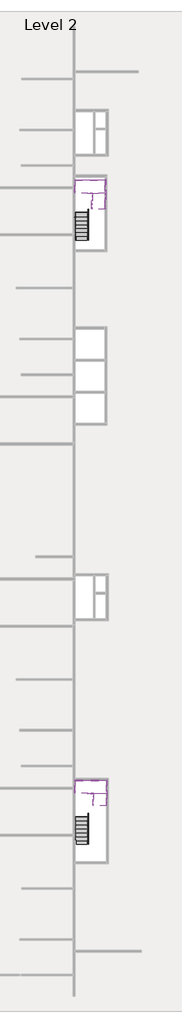
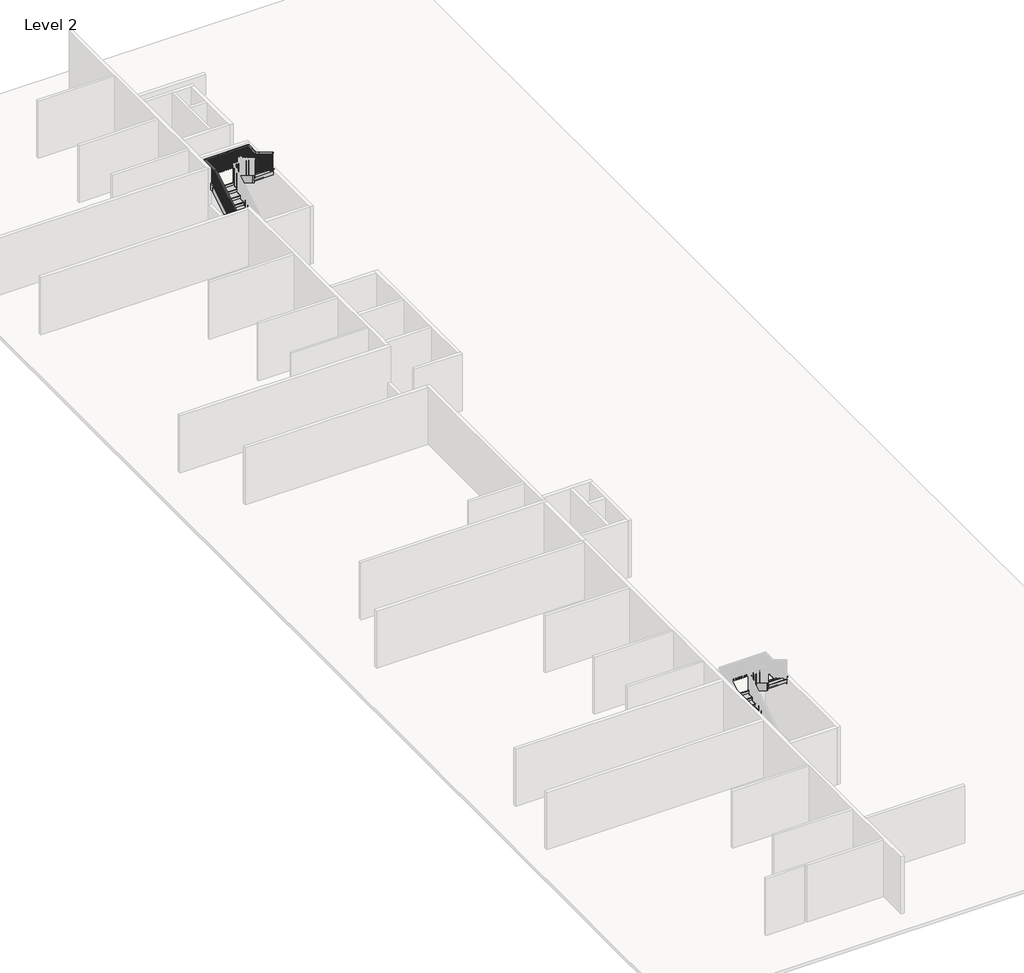
# One storey, part 8 of 8: 16 members, 4 stair flights, 2 slabs, 1 railing.
"""IFC4 building model written with IfcOpenShell, lengths in millimetres."""

from ifc_helpers import new_model, si_unit, frame, origin, place, context, project, spatial, polyline, outline, extrude, faceted_brep, transform, mapped, element, save
from components import non_monolithic_landing_5b8191bc, non_monolithic_landing_2a8916bf, stair_flight_17e69724, stair_flight_e6b75d85, stair_flight_770626d1, stair_flight_01bb6bd9

model = new_model("IFC4")

# Units and contexts
model_context = context("Model", 3, world=origin())
ifc_project = project(units=[si_unit("LENGTHUNIT", "METRE", prefix="MILLI")], contexts=[model_context])

# Site, building, storey
site = spatial("IfcSite", under=ifc_project)
building = spatial("IfcBuilding", under=site)
storey = spatial("IfcBuildingStorey", under=building, Name="Level 2", Elevation=28282.6172466)

# Members
placement = place(None, origin())
element("IfcMember", 1, ObjectType="Stringer - 2\" Width", at=placement, inside=storey, context=model_context, shape_type="SweptSolid", body=[
    extrude(outline(polyline([(-23154.3851539, 28282.6172466), (-23154.3851539, 28494.7317586), (-19467.0440987, 30729.4839133), (-19381.8896422, 30424.6839133), (-22916.2996422, 28282.6172466), (-23154.3851539, 28282.6172466)])), frame((-3668.2415084, 0.0, 0.0), z_axis=(1.0, 0.0, 0.0), x_axis=(0.0, 1.0, 0.0)), (0.0, 0.0, 1.0), 50.8),
])
element("IfcMember", 2, ObjectType="Stringer - 2\" Width", at=placement, inside=storey, context=model_context, shape_type="SweptSolid", body=[
    extrude(outline(polyline([(-23154.3851539, 28282.6172466), (-23154.3851539, 28494.7317586), (-19572.9851539, 30665.2772131), (-19572.9851539, 30308.8684516), (-22916.2996422, 28282.6172466), (-23154.3851539, 28282.6172466)])), frame((-2703.0415084, 0.0, 0.0), z_axis=(1.0, 0.0, 0.0), x_axis=(0.0, 1.0, 0.0)), (0.0, 0.0, 1.0), 50.8),
])
element("IfcMember", 3, ObjectType="Stringer - 2\" Width", at=placement, inside=storey, context=model_context, shape_type="SweptSolid", body=[
    extrude(outline(polyline([(-19297.9262092, 30729.4839133), (-19383.0806657, 30424.6839133), (-20360.3851539, 31016.9896637), (-20360.3851539, 31373.3984252), (-19297.9262092, 30729.4839133)])), frame((-1382.2415084, 0.0, 0.0), z_axis=(1.0, 0.0, 0.0), x_axis=(0.0, 1.0, 0.0)), (0.0, 0.0, 1.0), 50.8),
])
element("IfcMember", 4, ObjectType="Stringer - 2\" Width", at=placement, inside=storey, context=model_context, shape_type="SweptSolid", body=[
    extrude(outline(polyline([(-19522.1851539, 30865.3984252), (-19522.1851539, 30508.9896637), (-20360.3851539, 31016.9896637), (-20360.3851539, 31373.3984252), (-19522.1851539, 30865.3984252)])), frame((-2347.4415084, 0.0, 0.0), z_axis=(1.0, 0.0, 0.0), x_axis=(0.0, 1.0, 0.0)), (0.0, 0.0, 1.0), 50.8),
])
element("IfcMember", 5, ObjectType="Stringer - 2\" Width", at=placement, inside=storey, context=model_context, shape_type="Brep", body=[
    faceted_brep([(-1382.2415084, -19297.9262092, 30729.4839133), (-1331.4415084, -19297.9262092, 30729.4839133), (-1331.4415084, -18556.9851539, 30729.4839133), (-1382.2415084, -18607.7851539, 30729.4839133), (-1382.2415084, -19383.0806657, 30424.6839133), (-1382.2415084, -18607.7851539, 30424.6839133), (-1331.4415084, -19383.0806657, 30424.6839133), (-1331.4415084, -18556.9851539, 30424.6839133)], [[[0, 1, 2, 3]], [[4, 0, 3, 5]], [[6, 4, 5, 7]], [[1, 6, 7, 2]], [[1, 0, 4, 6]], [[2, 7, 5, 3]]]),
])
element("IfcMember", 6, ObjectType="Stringer - 2\" Width", at=placement, inside=storey, context=model_context, shape_type="SweptSolid", body=[
    extrude(outline(polyline([(-1331.4415084, -18556.9851539), (-1382.2415084, -18607.7851539), (-3617.4415084, -18607.7851539), (-3668.2415084, -18556.9851539), (-1331.4415084, -18556.9851539)])), frame((0.0, 0.0, 30424.6839133), z_axis=(0.0, 0.0, 1.0), x_axis=(1.0, 0.0, 0.0)), (0.0, 0.0, 1.0), 304.8),
])
element("IfcMember", 7, ObjectType="Stringer - 2\" Width", at=placement, inside=storey, context=model_context, shape_type="Brep", body=[
    faceted_brep([(-3617.4415084, -18607.7851539, 30729.4839133), (-3668.2415084, -18556.9851539, 30729.4839133), (-3668.2415084, -19467.0440987, 30729.4839133), (-3617.4415084, -19467.0440987, 30729.4839133), (-3617.4415084, -18607.7851539, 30424.6839133), (-3617.4415084, -19381.8896422, 30424.6839133), (-3668.2415084, -18556.9851539, 30424.6839133), (-3668.2415084, -19381.8896422, 30424.6839133)], [[[0, 1, 2, 3]], [[4, 0, 3, 5]], [[6, 4, 5, 7]], [[1, 6, 7, 2]], [[1, 0, 4, 6]], [[2, 7, 5, 3]]]),
])
element("IfcMember", 8, ObjectType="Stringer - 2\" Width", at=placement, inside=storey, context=model_context, shape_type="SweptSolid", body=[
    extrude(outline(polyline([(-2703.0415084, -19572.9851539), (-2703.0415084, -19522.1851539), (-2347.4415084, -19522.1851539), (-2347.4415084, -19572.9851539), (-2703.0415084, -19572.9851539)])), frame((0.0, 0.0, 30424.6839133), z_axis=(0.0, 0.0, 1.0), x_axis=(1.0, 0.0, 0.0)), (0.0, 0.0, 1.0), 304.8),
])
element("IfcMember", 9, ObjectType="Stringer - 2\" Width", at=placement, inside=storey, context=model_context, shape_type="SweptSolid", body=[
    extrude(outline(polyline([(19841.9216096, 28282.6172466), (19841.9216096, 28494.7317586), (23249.8626649, 30560.1505799), (23335.0171214, 30255.3505799), (20080.0071214, 28282.6172466), (19841.9216096, 28282.6172466)])), frame((-3668.2415084, 0.0, 0.0), z_axis=(1.0, 0.0, 0.0), x_axis=(0.0, 1.0, 0.0)), (0.0, 0.0, 1.0), 50.8),
])
element("IfcMember", 10, ObjectType="Stringer - 2\" Width", at=placement, inside=storey, context=model_context, shape_type="SweptSolid", body=[
    extrude(outline(polyline([(19841.9216096, 28282.6172466), (19841.9216096, 28494.7317586), (23143.9216096, 30495.9438798), (23143.9216096, 30139.5351183), (20080.0071214, 28282.6172466), (19841.9216096, 28282.6172466)])), frame((-2703.0415084, 0.0, 0.0), z_axis=(1.0, 0.0, 0.0), x_axis=(0.0, 1.0, 0.0)), (0.0, 0.0, 1.0), 50.8),
])
element("IfcMember", 11, ObjectType="Stringer - 2\" Width", at=placement, inside=storey, context=model_context, shape_type="SweptSolid", body=[
    extrude(outline(polyline([(23418.9805543, 30560.1505799), (23333.8260978, 30255.3505799), (22077.1216096, 31016.9896637), (22077.1216096, 31373.3984252), (23418.9805543, 30560.1505799)])), frame((-1483.8415084, 0.0, 0.0), z_axis=(1.0, 0.0, 0.0), x_axis=(0.0, 1.0, 0.0)), (0.0, 0.0, 1.0), 50.8),
])
element("IfcMember", 12, ObjectType="Stringer - 2\" Width", at=placement, inside=storey, context=model_context, shape_type="SweptSolid", body=[
    extrude(outline(polyline([(23194.7216096, 30696.0650919), (23194.7216096, 30339.6563304), (22077.1216096, 31016.9896637), (22077.1216096, 31373.3984252), (23194.7216096, 30696.0650919)])), frame((-2449.0415084, 0.0, 0.0), z_axis=(1.0, 0.0, 0.0), x_axis=(0.0, 1.0, 0.0)), (0.0, 0.0, 1.0), 50.8),
])
element("IfcMember", 13, ObjectType="Stringer - 2\" Width", at=placement, inside=storey, context=model_context, shape_type="Brep", body=[
    faceted_brep([(-1483.8415084, 23418.9805543, 30560.1505799), (-1433.0415084, 23418.9805543, 30560.1505799), (-1433.0415084, 24159.9216096, 30560.1505799), (-1483.8415084, 24109.1216096, 30560.1505799), (-1483.8415084, 23333.8260978, 30255.3505799), (-1483.8415084, 24109.1216096, 30255.3505799), (-1433.0415084, 23333.8260978, 30255.3505799), (-1433.0415084, 24159.9216096, 30255.3505799)], [[[0, 1, 2, 3]], [[4, 0, 3, 5]], [[6, 4, 5, 7]], [[1, 6, 7, 2]], [[1, 0, 4, 6]], [[2, 7, 5, 3]]]),
])
element("IfcMember", 14, ObjectType="Stringer - 2\" Width", at=placement, inside=storey, context=model_context, shape_type="SweptSolid", body=[
    extrude(outline(polyline([(-1433.0415084, 24159.9216096), (-1483.8415084, 24109.1216096), (-3617.4415084, 24109.1216096), (-3668.2415084, 24159.9216096), (-1433.0415084, 24159.9216096)])), frame((0.0, 0.0, 30255.3505799), z_axis=(0.0, 0.0, 1.0), x_axis=(1.0, 0.0, 0.0)), (0.0, 0.0, 1.0), 304.8),
])
element("IfcMember", 15, ObjectType="Stringer - 2\" Width", at=placement, inside=storey, context=model_context, shape_type="Brep", body=[
    faceted_brep([(-3617.4415084, 24109.1216096, 30560.1505799), (-3668.2415084, 24159.9216096, 30560.1505799), (-3668.2415084, 23249.8626649, 30560.1505799), (-3617.4415084, 23249.8626649, 30560.1505799), (-3617.4415084, 24109.1216096, 30255.3505799), (-3617.4415084, 23335.0171214, 30255.3505799), (-3668.2415084, 24159.9216096, 30255.3505799), (-3668.2415084, 23335.0171214, 30255.3505799)], [[[0, 1, 2, 3]], [[4, 0, 3, 5]], [[6, 4, 5, 7]], [[1, 6, 7, 2]], [[1, 0, 4, 6]], [[2, 7, 5, 3]]]),
])
element("IfcMember", 16, ObjectType="Stringer - 2\" Width", at=placement, inside=storey, context=model_context, shape_type="SweptSolid", body=[
    extrude(outline(polyline([(-2703.0415084, 23143.9216096), (-2703.0415084, 23194.7216096), (-2449.0415084, 23194.7216096), (-2449.0415084, 23143.9216096), (-2703.0415084, 23143.9216096)])), frame((0.0, 0.0, 30255.3505799), z_axis=(0.0, 0.0, 1.0), x_axis=(1.0, 0.0, 0.0)), (0.0, 0.0, 1.0), 304.8),
])

# Railing
element("IfcRailing", 17, ObjectType="Handrail - Rectangular", at=placement, inside=storey, context=model_context, shape_type="SolidModel", body=[
    faceted_brep([(-3617.4415084, 19841.9216096, 29366.3505799), (-3617.4415084, 19841.9216096, 29306.9491197), (-3566.6415084, 19841.9216096, 29306.9491197), (-3566.6415084, 19841.9216096, 29366.3505799), (-3617.4415084, 23194.7216096, 31398.3505799), (-3617.4415084, 23208.914019, 31347.5505799), (-3566.6415084, 23208.914019, 31347.5505799), (-3566.6415084, 23194.7216096, 31398.3505799), (-3617.4415084, 24109.1216096, 31398.3505799), (-3617.4415084, 24109.1216096, 31347.5505799), (-3566.6415084, 24058.3216096, 31347.5505799), (-3566.6415084, 24058.3216096, 31398.3505799), (-1483.8415084, 24109.1216096, 31398.3505799), (-1483.8415084, 24109.1216096, 31347.5505799), (-1534.6415084, 24058.3216096, 31347.5505799), (-1534.6415084, 24058.3216096, 31398.3505799), (-1483.8415084, 23474.1216096, 31398.3505799), (-1483.8415084, 23459.9292002, 31347.5505799), (-1534.6415084, 23459.9292002, 31347.5505799), (-1534.6415084, 23474.1216096, 31398.3505799), (-1483.8415084, 23194.7216096, 31567.6839133), (-1483.8415084, 23168.3918824, 31524.2398634), (-1534.6415084, 23168.3918824, 31524.2398634), (-1534.6415084, 23194.7216096, 31567.6839133), (-1483.8415084, 22077.1216096, 32245.0172466), (-1534.6415084, 22077.1216096, 32245.0172466), (-1534.6415084, 22077.1216096, 32185.6157863), (-1483.8415084, 22077.1216096, 32185.6157863)], [[[0, 1, 2, 3]], [[1, 0, 4, 5]], [[2, 1, 5, 6]], [[3, 2, 6, 7]], [[0, 3, 7, 4]], [[5, 4, 8, 9]], [[6, 5, 9, 10]], [[7, 6, 10, 11]], [[4, 7, 11, 8]], [[9, 8, 12, 13]], [[10, 9, 13, 14]], [[11, 10, 14, 15]], [[8, 11, 15, 12]], [[13, 12, 16, 17]], [[14, 13, 17, 18]], [[15, 14, 18, 19]], [[12, 15, 19, 16]], [[17, 16, 20, 21]], [[18, 17, 21, 22]], [[19, 18, 22, 23]], [[16, 19, 23, 20]], [[24, 25, 26, 27]], [[21, 20, 24, 27]], [[22, 21, 27, 26]], [[23, 22, 26, 25]], [[20, 23, 25, 24]]]),
    extrude(outline(polyline([(22188.2466096, 32118.2673015), (22188.2466096, 31161.2839133), (22169.1966096, 31161.2839133), (22169.1966096, 32129.812756), (22188.2466096, 32118.2673015)])), frame((-1518.7665084, 0.0, 0.0), z_axis=(1.0, 0.0, 0.0), x_axis=(0.0, 1.0, 0.0)), (0.0, 0.0, 1.0), 19.05),
    extrude(outline(polyline([(22289.8466096, 32056.6915439), (22289.8466096, 31161.2839133), (22270.7966096, 31161.2839133), (22270.7966096, 32068.2369985), (22289.8466096, 32056.6915439)])), frame((-1518.7665084, 0.0, 0.0), z_axis=(1.0, 0.0, 0.0), x_axis=(0.0, 1.0, 0.0)), (0.0, 0.0, 1.0), 19.05),
    extrude(outline(polyline([(22391.4466096, 31995.1157863), (22391.4466096, 30991.9505799), (22372.3966096, 30991.9505799), (22372.3966096, 32006.6612409), (22391.4466096, 31995.1157863)])), frame((-1518.7665084, 0.0, 0.0), z_axis=(1.0, 0.0, 0.0), x_axis=(0.0, 1.0, 0.0)), (0.0, 0.0, 1.0), 19.05),
    extrude(outline(polyline([(22493.0466096, 31933.5400288), (22493.0466096, 30991.9505799), (22473.9966096, 30991.9505799), (22473.9966096, 31945.0854833), (22493.0466096, 31933.5400288)])), frame((-1518.7665084, 0.0, 0.0), z_axis=(1.0, 0.0, 0.0), x_axis=(0.0, 1.0, 0.0)), (0.0, 0.0, 1.0), 19.05),
    extrude(outline(polyline([(22594.6466096, 31871.9642712), (22594.6466096, 30991.9505799), (22575.5966096, 30991.9505799), (22575.5966096, 31883.5097257), (22594.6466096, 31871.9642712)])), frame((-1518.7665084, 0.0, 0.0), z_axis=(1.0, 0.0, 0.0), x_axis=(0.0, 1.0, 0.0)), (0.0, 0.0, 1.0), 19.05),
    extrude(outline(polyline([(22696.2466096, 31810.3885136), (22696.2466096, 30822.6172466), (22677.1966096, 30822.6172466), (22677.1966096, 31821.9339682), (22696.2466096, 31810.3885136)])), frame((-1518.7665084, 0.0, 0.0), z_axis=(1.0, 0.0, 0.0), x_axis=(0.0, 1.0, 0.0)), (0.0, 0.0, 1.0), 19.05),
    extrude(outline(polyline([(22797.8466096, 31748.812756), (22797.8466096, 30822.6172466), (22778.7966096, 30822.6172466), (22778.7966096, 31760.3582106), (22797.8466096, 31748.812756)])), frame((-1518.7665084, 0.0, 0.0), z_axis=(1.0, 0.0, 0.0), x_axis=(0.0, 1.0, 0.0)), (0.0, 0.0, 1.0), 19.05),
    extrude(outline(polyline([(22899.4466096, 31687.2369985), (22899.4466096, 30822.6172466), (22880.3966096, 30822.6172466), (22880.3966096, 31698.782453), (22899.4466096, 31687.2369985)])), frame((-1518.7665084, 0.0, 0.0), z_axis=(1.0, 0.0, 0.0), x_axis=(0.0, 1.0, 0.0)), (0.0, 0.0, 1.0), 19.05),
    extrude(outline(polyline([(23001.0466096, 31625.6612409), (23001.0466096, 30653.2839133), (22981.9966096, 30653.2839133), (22981.9966096, 31637.2066954), (23001.0466096, 31625.6612409)])), frame((-1518.7665084, 0.0, 0.0), z_axis=(1.0, 0.0, 0.0), x_axis=(0.0, 1.0, 0.0)), (0.0, 0.0, 1.0), 19.05),
    extrude(outline(polyline([(23102.6466096, 31564.0854833), (23102.6466096, 30653.2839133), (23083.5966096, 30653.2839133), (23083.5966096, 31575.6309379), (23102.6466096, 31564.0854833)])), frame((-1518.7665084, 0.0, 0.0), z_axis=(1.0, 0.0, 0.0), x_axis=(0.0, 1.0, 0.0)), (0.0, 0.0, 1.0), 19.05),
    extrude(outline(polyline([(23280.4466096, 31456.3279076), (23280.4466096, 30483.9505799), (23261.3966096, 30483.9505799), (23261.3966096, 31467.8733621), (23280.4466096, 31456.3279076)])), frame((-1518.7665084, 0.0, 0.0), z_axis=(1.0, 0.0, 0.0), x_axis=(0.0, 1.0, 0.0)), (0.0, 0.0, 1.0), 19.05),
    extrude(outline(polyline([(23382.0466096, 31394.75215), (23382.0466096, 30483.9505799), (23362.9966096, 30483.9505799), (23362.9966096, 31406.2976045), (23382.0466096, 31394.75215)])), frame((-1518.7665084, 0.0, 0.0), z_axis=(1.0, 0.0, 0.0), x_axis=(0.0, 1.0, 0.0)), (0.0, 0.0, 1.0), 19.05),
    extrude(outline(polyline([(-1499.7165084, 23483.6466096), (-1499.7165084, 23464.5966096), (-1518.7665084, 23464.5966096), (-1518.7665084, 23483.6466096), (-1499.7165084, 23483.6466096)])), frame((0.0, 0.0, 30483.9505799), z_axis=(0.0, 0.0, 1.0), x_axis=(1.0, 0.0, 0.0)), (0.0, 0.0, 1.0), 863.6),
    extrude(outline(polyline([(-1499.7165084, 23585.2466096), (-1499.7165084, 23566.1966096), (-1518.7665084, 23566.1966096), (-1518.7665084, 23585.2466096), (-1499.7165084, 23585.2466096)])), frame((0.0, 0.0, 30483.9505799), z_axis=(0.0, 0.0, 1.0), x_axis=(1.0, 0.0, 0.0)), (0.0, 0.0, 1.0), 863.6),
    extrude(outline(polyline([(-1499.7165084, 23686.8466096), (-1499.7165084, 23667.7966096), (-1518.7665084, 23667.7966096), (-1518.7665084, 23686.8466096), (-1499.7165084, 23686.8466096)])), frame((0.0, 0.0, 30483.9505799), z_axis=(0.0, 0.0, 1.0), x_axis=(1.0, 0.0, 0.0)), (0.0, 0.0, 1.0), 863.6),
    extrude(outline(polyline([(-1499.7165084, 23788.4466096), (-1499.7165084, 23769.3966096), (-1518.7665084, 23769.3966096), (-1518.7665084, 23788.4466096), (-1499.7165084, 23788.4466096)])), frame((0.0, 0.0, 30483.9505799), z_axis=(0.0, 0.0, 1.0), x_axis=(1.0, 0.0, 0.0)), (0.0, 0.0, 1.0), 863.6),
    extrude(outline(polyline([(-1499.7165084, 23890.0466096), (-1499.7165084, 23870.9966096), (-1518.7665084, 23870.9966096), (-1518.7665084, 23890.0466096), (-1499.7165084, 23890.0466096)])), frame((0.0, 0.0, 30483.9505799), z_axis=(0.0, 0.0, 1.0), x_axis=(1.0, 0.0, 0.0)), (0.0, 0.0, 1.0), 863.6),
    extrude(outline(polyline([(-1499.7165084, 23991.6466096), (-1499.7165084, 23972.5966096), (-1518.7665084, 23972.5966096), (-1518.7665084, 23991.6466096), (-1499.7165084, 23991.6466096)])), frame((0.0, 0.0, 30483.9505799), z_axis=(0.0, 0.0, 1.0), x_axis=(1.0, 0.0, 0.0)), (0.0, 0.0, 1.0), 863.6),
    extrude(outline(polyline([(-1569.5665084, 24093.2466096), (-1550.5165084, 24093.2466096), (-1550.5165084, 24074.1966096), (-1569.5665084, 24074.1966096), (-1569.5665084, 24093.2466096)])), frame((0.0, 0.0, 30483.9505799), z_axis=(0.0, 0.0, 1.0), x_axis=(1.0, 0.0, 0.0)), (0.0, 0.0, 1.0), 863.6),
    extrude(outline(polyline([(-1671.1665084, 24093.2466096), (-1652.1165084, 24093.2466096), (-1652.1165084, 24074.1966096), (-1671.1665084, 24074.1966096), (-1671.1665084, 24093.2466096)])), frame((0.0, 0.0, 30483.9505799), z_axis=(0.0, 0.0, 1.0), x_axis=(1.0, 0.0, 0.0)), (0.0, 0.0, 1.0), 863.6),
    extrude(outline(polyline([(-1772.7665084, 24093.2466096), (-1753.7165084, 24093.2466096), (-1753.7165084, 24074.1966096), (-1772.7665084, 24074.1966096), (-1772.7665084, 24093.2466096)])), frame((0.0, 0.0, 30483.9505799), z_axis=(0.0, 0.0, 1.0), x_axis=(1.0, 0.0, 0.0)), (0.0, 0.0, 1.0), 863.6),
    extrude(outline(polyline([(-1874.3665084, 24093.2466096), (-1855.3165084, 24093.2466096), (-1855.3165084, 24074.1966096), (-1874.3665084, 24074.1966096), (-1874.3665084, 24093.2466096)])), frame((0.0, 0.0, 30483.9505799), z_axis=(0.0, 0.0, 1.0), x_axis=(1.0, 0.0, 0.0)), (0.0, 0.0, 1.0), 863.6),
    extrude(outline(polyline([(-1975.9665084, 24093.2466096), (-1956.9165084, 24093.2466096), (-1956.9165084, 24074.1966096), (-1975.9665084, 24074.1966096), (-1975.9665084, 24093.2466096)])), frame((0.0, 0.0, 30483.9505799), z_axis=(0.0, 0.0, 1.0), x_axis=(1.0, 0.0, 0.0)), (0.0, 0.0, 1.0), 863.6),
    extrude(outline(polyline([(-2077.5665084, 24093.2466096), (-2058.5165084, 24093.2466096), (-2058.5165084, 24074.1966096), (-2077.5665084, 24074.1966096), (-2077.5665084, 24093.2466096)])), frame((0.0, 0.0, 30483.9505799), z_axis=(0.0, 0.0, 1.0), x_axis=(1.0, 0.0, 0.0)), (0.0, 0.0, 1.0), 863.6),
    extrude(outline(polyline([(-2179.1665084, 24093.2466096), (-2160.1165084, 24093.2466096), (-2160.1165084, 24074.1966096), (-2179.1665084, 24074.1966096), (-2179.1665084, 24093.2466096)])), frame((0.0, 0.0, 30483.9505799), z_axis=(0.0, 0.0, 1.0), x_axis=(1.0, 0.0, 0.0)), (0.0, 0.0, 1.0), 863.6),
    extrude(outline(polyline([(-2280.7665084, 24093.2466096), (-2261.7165084, 24093.2466096), (-2261.7165084, 24074.1966096), (-2280.7665084, 24074.1966096), (-2280.7665084, 24093.2466096)])), frame((0.0, 0.0, 30483.9505799), z_axis=(0.0, 0.0, 1.0), x_axis=(1.0, 0.0, 0.0)), (0.0, 0.0, 1.0), 863.6),
    extrude(outline(polyline([(-2382.3665084, 24093.2466096), (-2363.3165084, 24093.2466096), (-2363.3165084, 24074.1966096), (-2382.3665084, 24074.1966096), (-2382.3665084, 24093.2466096)])), frame((0.0, 0.0, 30483.9505799), z_axis=(0.0, 0.0, 1.0), x_axis=(1.0, 0.0, 0.0)), (0.0, 0.0, 1.0), 863.6),
    extrude(outline(polyline([(-2483.9665084, 24093.2466096), (-2464.9165084, 24093.2466096), (-2464.9165084, 24074.1966096), (-2483.9665084, 24074.1966096), (-2483.9665084, 24093.2466096)])), frame((0.0, 0.0, 30483.9505799), z_axis=(0.0, 0.0, 1.0), x_axis=(1.0, 0.0, 0.0)), (0.0, 0.0, 1.0), 863.6),
    extrude(outline(polyline([(-2585.5665084, 24093.2466096), (-2566.5165084, 24093.2466096), (-2566.5165084, 24074.1966096), (-2585.5665084, 24074.1966096), (-2585.5665084, 24093.2466096)])), frame((0.0, 0.0, 30483.9505799), z_axis=(0.0, 0.0, 1.0), x_axis=(1.0, 0.0, 0.0)), (0.0, 0.0, 1.0), 863.6),
    extrude(outline(polyline([(-2687.1665084, 24093.2466096), (-2668.1165084, 24093.2466096), (-2668.1165084, 24074.1966096), (-2687.1665084, 24074.1966096), (-2687.1665084, 24093.2466096)])), frame((0.0, 0.0, 30483.9505799), z_axis=(0.0, 0.0, 1.0), x_axis=(1.0, 0.0, 0.0)), (0.0, 0.0, 1.0), 863.6),
    extrude(outline(polyline([(-2788.7665084, 24093.2466096), (-2769.7165084, 24093.2466096), (-2769.7165084, 24074.1966096), (-2788.7665084, 24074.1966096), (-2788.7665084, 24093.2466096)])), frame((0.0, 0.0, 30483.9505799), z_axis=(0.0, 0.0, 1.0), x_axis=(1.0, 0.0, 0.0)), (0.0, 0.0, 1.0), 863.6),
    extrude(outline(polyline([(-2890.3665084, 24093.2466096), (-2871.3165084, 24093.2466096), (-2871.3165084, 24074.1966096), (-2890.3665084, 24074.1966096), (-2890.3665084, 24093.2466096)])), frame((0.0, 0.0, 30483.9505799), z_axis=(0.0, 0.0, 1.0), x_axis=(1.0, 0.0, 0.0)), (0.0, 0.0, 1.0), 863.6),
    extrude(outline(polyline([(-2991.9665084, 24093.2466096), (-2972.9165084, 24093.2466096), (-2972.9165084, 24074.1966096), (-2991.9665084, 24074.1966096), (-2991.9665084, 24093.2466096)])), frame((0.0, 0.0, 30483.9505799), z_axis=(0.0, 0.0, 1.0), x_axis=(1.0, 0.0, 0.0)), (0.0, 0.0, 1.0), 863.6),
    extrude(outline(polyline([(-3093.5665084, 24093.2466096), (-3074.5165084, 24093.2466096), (-3074.5165084, 24074.1966096), (-3093.5665084, 24074.1966096), (-3093.5665084, 24093.2466096)])), frame((0.0, 0.0, 30483.9505799), z_axis=(0.0, 0.0, 1.0), x_axis=(1.0, 0.0, 0.0)), (0.0, 0.0, 1.0), 863.6),
    extrude(outline(polyline([(-3195.1665084, 24093.2466096), (-3176.1165084, 24093.2466096), (-3176.1165084, 24074.1966096), (-3195.1665084, 24074.1966096), (-3195.1665084, 24093.2466096)])), frame((0.0, 0.0, 30483.9505799), z_axis=(0.0, 0.0, 1.0), x_axis=(1.0, 0.0, 0.0)), (0.0, 0.0, 1.0), 863.6),
    extrude(outline(polyline([(-3296.7665084, 24093.2466096), (-3277.7165084, 24093.2466096), (-3277.7165084, 24074.1966096), (-3296.7665084, 24074.1966096), (-3296.7665084, 24093.2466096)])), frame((0.0, 0.0, 30483.9505799), z_axis=(0.0, 0.0, 1.0), x_axis=(1.0, 0.0, 0.0)), (0.0, 0.0, 1.0), 863.6),
    extrude(outline(polyline([(-3398.3665084, 24093.2466096), (-3379.3165084, 24093.2466096), (-3379.3165084, 24074.1966096), (-3398.3665084, 24074.1966096), (-3398.3665084, 24093.2466096)])), frame((0.0, 0.0, 30483.9505799), z_axis=(0.0, 0.0, 1.0), x_axis=(1.0, 0.0, 0.0)), (0.0, 0.0, 1.0), 863.6),
    extrude(outline(polyline([(-3499.9665084, 24093.2466096), (-3480.9165084, 24093.2466096), (-3480.9165084, 24074.1966096), (-3499.9665084, 24074.1966096), (-3499.9665084, 24093.2466096)])), frame((0.0, 0.0, 30483.9505799), z_axis=(0.0, 0.0, 1.0), x_axis=(1.0, 0.0, 0.0)), (0.0, 0.0, 1.0), 863.6),
    extrude(outline(polyline([(-3601.5665084, 23997.9966096), (-3601.5665084, 24017.0466096), (-3582.5165084, 24017.0466096), (-3582.5165084, 23997.9966096), (-3601.5665084, 23997.9966096)])), frame((0.0, 0.0, 30483.9505799), z_axis=(0.0, 0.0, 1.0), x_axis=(1.0, 0.0, 0.0)), (0.0, 0.0, 1.0), 863.6),
    extrude(outline(polyline([(-3601.5665084, 23896.3966096), (-3601.5665084, 23915.4466096), (-3582.5165084, 23915.4466096), (-3582.5165084, 23896.3966096), (-3601.5665084, 23896.3966096)])), frame((0.0, 0.0, 30483.9505799), z_axis=(0.0, 0.0, 1.0), x_axis=(1.0, 0.0, 0.0)), (0.0, 0.0, 1.0), 863.6),
    extrude(outline(polyline([(-3601.5665084, 23794.7966096), (-3601.5665084, 23813.8466096), (-3582.5165084, 23813.8466096), (-3582.5165084, 23794.7966096), (-3601.5665084, 23794.7966096)])), frame((0.0, 0.0, 30483.9505799), z_axis=(0.0, 0.0, 1.0), x_axis=(1.0, 0.0, 0.0)), (0.0, 0.0, 1.0), 863.6),
    extrude(outline(polyline([(-3601.5665084, 23693.1966096), (-3601.5665084, 23712.2466096), (-3582.5165084, 23712.2466096), (-3582.5165084, 23693.1966096), (-3601.5665084, 23693.1966096)])), frame((0.0, 0.0, 30483.9505799), z_axis=(0.0, 0.0, 1.0), x_axis=(1.0, 0.0, 0.0)), (0.0, 0.0, 1.0), 863.6),
    extrude(outline(polyline([(-3601.5665084, 23591.5966096), (-3601.5665084, 23610.6466096), (-3582.5165084, 23610.6466096), (-3582.5165084, 23591.5966096), (-3601.5665084, 23591.5966096)])), frame((0.0, 0.0, 30483.9505799), z_axis=(0.0, 0.0, 1.0), x_axis=(1.0, 0.0, 0.0)), (0.0, 0.0, 1.0), 863.6),
    extrude(outline(polyline([(-3601.5665084, 23489.9966096), (-3601.5665084, 23509.0466096), (-3582.5165084, 23509.0466096), (-3582.5165084, 23489.9966096), (-3601.5665084, 23489.9966096)])), frame((0.0, 0.0, 30483.9505799), z_axis=(0.0, 0.0, 1.0), x_axis=(1.0, 0.0, 0.0)), (0.0, 0.0, 1.0), 863.6),
    extrude(outline(polyline([(-3601.5665084, 23388.3966096), (-3601.5665084, 23407.4466096), (-3582.5165084, 23407.4466096), (-3582.5165084, 23388.3966096), (-3601.5665084, 23388.3966096)])), frame((0.0, 0.0, 30483.9505799), z_axis=(0.0, 0.0, 1.0), x_axis=(1.0, 0.0, 0.0)), (0.0, 0.0, 1.0), 863.6),
    extrude(outline(polyline([(-3601.5665084, 23286.7966096), (-3601.5665084, 23305.8466096), (-3582.5165084, 23305.8466096), (-3582.5165084, 23286.7966096), (-3601.5665084, 23286.7966096)])), frame((0.0, 0.0, 30483.9505799), z_axis=(0.0, 0.0, 1.0), x_axis=(1.0, 0.0, 0.0)), (0.0, 0.0, 1.0), 863.6),
    extrude(outline(polyline([(23102.6466096, 31283.1460894), (23102.6466096, 30314.6172466), (23083.5966096, 30314.6172466), (23083.5966096, 31271.6006348), (23102.6466096, 31283.1460894)])), frame((-3601.5665084, 0.0, 0.0), z_axis=(1.0, 0.0, 0.0), x_axis=(0.0, 1.0, 0.0)), (0.0, 0.0, 1.0), 19.05),
    extrude(outline(polyline([(23001.0466096, 31221.5703318), (23001.0466096, 30314.6172466), (22981.9966096, 30314.6172466), (22981.9966096, 31210.0248773), (23001.0466096, 31221.5703318)])), frame((-3601.5665084, 0.0, 0.0), z_axis=(1.0, 0.0, 0.0), x_axis=(0.0, 1.0, 0.0)), (0.0, 0.0, 1.0), 19.05),
    extrude(outline(polyline([(22899.4466096, 31159.9945742), (22899.4466096, 30145.2839133), (22880.3966096, 30145.2839133), (22880.3966096, 31148.4491197), (22899.4466096, 31159.9945742)])), frame((-3601.5665084, 0.0, 0.0), z_axis=(1.0, 0.0, 0.0), x_axis=(0.0, 1.0, 0.0)), (0.0, 0.0, 1.0), 19.05),
    extrude(outline(polyline([(22797.8466096, 31098.4188167), (22797.8466096, 30145.2839133), (22778.7966096, 30145.2839133), (22778.7966096, 31086.8733621), (22797.8466096, 31098.4188167)])), frame((-3601.5665084, 0.0, 0.0), z_axis=(1.0, 0.0, 0.0), x_axis=(0.0, 1.0, 0.0)), (0.0, 0.0, 1.0), 19.05),
    extrude(outline(polyline([(22696.2466096, 31036.8430591), (22696.2466096, 30145.2839133), (22677.1966096, 30145.2839133), (22677.1966096, 31025.2976045), (22696.2466096, 31036.8430591)])), frame((-3601.5665084, 0.0, 0.0), z_axis=(1.0, 0.0, 0.0), x_axis=(0.0, 1.0, 0.0)), (0.0, 0.0, 1.0), 19.05),
    extrude(outline(polyline([(22594.6466096, 30975.2673015), (22594.6466096, 29975.9505799), (22575.5966096, 29975.9505799), (22575.5966096, 30963.721847), (22594.6466096, 30975.2673015)])), frame((-3601.5665084, 0.0, 0.0), z_axis=(1.0, 0.0, 0.0), x_axis=(0.0, 1.0, 0.0)), (0.0, 0.0, 1.0), 19.05),
    extrude(outline(polyline([(22493.0466096, 30913.6915439), (22493.0466096, 29975.9505799), (22473.9966096, 29975.9505799), (22473.9966096, 30902.1460894), (22493.0466096, 30913.6915439)])), frame((-3601.5665084, 0.0, 0.0), z_axis=(1.0, 0.0, 0.0), x_axis=(0.0, 1.0, 0.0)), (0.0, 0.0, 1.0), 19.05),
    extrude(outline(polyline([(22391.4466096, 30852.1157863), (22391.4466096, 29975.9505799), (22372.3966096, 29975.9505799), (22372.3966096, 30840.5703318), (22391.4466096, 30852.1157863)])), frame((-3601.5665084, 0.0, 0.0), z_axis=(1.0, 0.0, 0.0), x_axis=(0.0, 1.0, 0.0)), (0.0, 0.0, 1.0), 19.05),
    extrude(outline(polyline([(22289.8466096, 30790.5400288), (22289.8466096, 29806.6172466), (22270.7966096, 29806.6172466), (22270.7966096, 30778.9945742), (22289.8466096, 30790.5400288)])), frame((-3601.5665084, 0.0, 0.0), z_axis=(1.0, 0.0, 0.0), x_axis=(0.0, 1.0, 0.0)), (0.0, 0.0, 1.0), 19.05),
    extrude(outline(polyline([(22188.2466096, 30728.9642712), (22188.2466096, 29806.6172466), (22169.1966096, 29806.6172466), (22169.1966096, 30717.4188167), (22188.2466096, 30728.9642712)])), frame((-3601.5665084, 0.0, 0.0), z_axis=(1.0, 0.0, 0.0), x_axis=(0.0, 1.0, 0.0)), (0.0, 0.0, 1.0), 19.05),
    extrude(outline(polyline([(22086.6466096, 30667.3885136), (22086.6466096, 29806.6172466), (22067.5966096, 29806.6172466), (22067.5966096, 30655.8430591), (22086.6466096, 30667.3885136)])), frame((-3601.5665084, 0.0, 0.0), z_axis=(1.0, 0.0, 0.0), x_axis=(0.0, 1.0, 0.0)), (0.0, 0.0, 1.0), 19.05),
    extrude(outline(polyline([(21985.0466096, 30605.812756), (21985.0466096, 29637.2839133), (21965.9966096, 29637.2839133), (21965.9966096, 30594.2673015), (21985.0466096, 30605.812756)])), frame((-3601.5665084, 0.0, 0.0), z_axis=(1.0, 0.0, 0.0), x_axis=(0.0, 1.0, 0.0)), (0.0, 0.0, 1.0), 19.05),
    extrude(outline(polyline([(21883.4466096, 30544.2369985), (21883.4466096, 29637.2839133), (21864.3966096, 29637.2839133), (21864.3966096, 30532.6915439), (21883.4466096, 30544.2369985)])), frame((-3601.5665084, 0.0, 0.0), z_axis=(1.0, 0.0, 0.0), x_axis=(0.0, 1.0, 0.0)), (0.0, 0.0, 1.0), 19.05),
    extrude(outline(polyline([(21781.8466096, 30482.6612409), (21781.8466096, 29467.9505799), (21762.7966096, 29467.9505799), (21762.7966096, 30471.1157863), (21781.8466096, 30482.6612409)])), frame((-3601.5665084, 0.0, 0.0), z_axis=(1.0, 0.0, 0.0), x_axis=(0.0, 1.0, 0.0)), (0.0, 0.0, 1.0), 19.05),
    extrude(outline(polyline([(21680.2466096, 30421.0854833), (21680.2466096, 29467.9505799), (21661.1966096, 29467.9505799), (21661.1966096, 30409.5400288), (21680.2466096, 30421.0854833)])), frame((-3601.5665084, 0.0, 0.0), z_axis=(1.0, 0.0, 0.0), x_axis=(0.0, 1.0, 0.0)), (0.0, 0.0, 1.0), 19.05),
    extrude(outline(polyline([(21578.6466096, 30359.5097257), (21578.6466096, 29467.9505799), (21559.5966096, 29467.9505799), (21559.5966096, 30347.9642712), (21578.6466096, 30359.5097257)])), frame((-3601.5665084, 0.0, 0.0), z_axis=(1.0, 0.0, 0.0), x_axis=(0.0, 1.0, 0.0)), (0.0, 0.0, 1.0), 19.05),
    extrude(outline(polyline([(21477.0466096, 30297.9339682), (21477.0466096, 29298.6172466), (21457.9966096, 29298.6172466), (21457.9966096, 30286.3885136), (21477.0466096, 30297.9339682)])), frame((-3601.5665084, 0.0, 0.0), z_axis=(1.0, 0.0, 0.0), x_axis=(0.0, 1.0, 0.0)), (0.0, 0.0, 1.0), 19.05),
    extrude(outline(polyline([(21375.4466096, 30236.3582106), (21375.4466096, 29298.6172466), (21356.3966096, 29298.6172466), (21356.3966096, 30224.812756), (21375.4466096, 30236.3582106)])), frame((-3601.5665084, 0.0, 0.0), z_axis=(1.0, 0.0, 0.0), x_axis=(0.0, 1.0, 0.0)), (0.0, 0.0, 1.0), 19.05),
    extrude(outline(polyline([(21273.8466096, 30174.782453), (21273.8466096, 29298.6172466), (21254.7966096, 29298.6172466), (21254.7966096, 30163.2369985), (21273.8466096, 30174.782453)])), frame((-3601.5665084, 0.0, 0.0), z_axis=(1.0, 0.0, 0.0), x_axis=(0.0, 1.0, 0.0)), (0.0, 0.0, 1.0), 19.05),
    extrude(outline(polyline([(21172.2466096, 30113.2066954), (21172.2466096, 29129.2839133), (21153.1966096, 29129.2839133), (21153.1966096, 30101.6612409), (21172.2466096, 30113.2066954)])), frame((-3601.5665084, 0.0, 0.0), z_axis=(1.0, 0.0, 0.0), x_axis=(0.0, 1.0, 0.0)), (0.0, 0.0, 1.0), 19.05),
    extrude(outline(polyline([(21070.6466096, 30051.6309379), (21070.6466096, 29129.2839133), (21051.5966096, 29129.2839133), (21051.5966096, 30040.0854833), (21070.6466096, 30051.6309379)])), frame((-3601.5665084, 0.0, 0.0), z_axis=(1.0, 0.0, 0.0), x_axis=(0.0, 1.0, 0.0)), (0.0, 0.0, 1.0), 19.05),
    extrude(outline(polyline([(20969.0466096, 29990.0551803), (20969.0466096, 29129.2839133), (20949.9966096, 29129.2839133), (20949.9966096, 29978.5097257), (20969.0466096, 29990.0551803)])), frame((-3601.5665084, 0.0, 0.0), z_axis=(1.0, 0.0, 0.0), x_axis=(0.0, 1.0, 0.0)), (0.0, 0.0, 1.0), 19.05),
    extrude(outline(polyline([(20867.4466096, 29928.4794227), (20867.4466096, 28959.9505799), (20848.3966096, 28959.9505799), (20848.3966096, 29916.9339682), (20867.4466096, 29928.4794227)])), frame((-3601.5665084, 0.0, 0.0), z_axis=(1.0, 0.0, 0.0), x_axis=(0.0, 1.0, 0.0)), (0.0, 0.0, 1.0), 19.05),
    extrude(outline(polyline([(20765.8466096, 29866.9036651), (20765.8466096, 28959.9505799), (20746.7966096, 28959.9505799), (20746.7966096, 29855.3582106), (20765.8466096, 29866.9036651)])), frame((-3601.5665084, 0.0, 0.0), z_axis=(1.0, 0.0, 0.0), x_axis=(0.0, 1.0, 0.0)), (0.0, 0.0, 1.0), 19.05),
    extrude(outline(polyline([(20664.2466096, 29805.3279076), (20664.2466096, 28790.6172466), (20645.1966096, 28790.6172466), (20645.1966096, 29793.782453), (20664.2466096, 29805.3279076)])), frame((-3601.5665084, 0.0, 0.0), z_axis=(1.0, 0.0, 0.0), x_axis=(0.0, 1.0, 0.0)), (0.0, 0.0, 1.0), 19.05),
    extrude(outline(polyline([(20562.6466096, 29743.75215), (20562.6466096, 28790.6172466), (20543.5966096, 28790.6172466), (20543.5966096, 29732.2066954), (20562.6466096, 29743.75215)])), frame((-3601.5665084, 0.0, 0.0), z_axis=(1.0, 0.0, 0.0), x_axis=(0.0, 1.0, 0.0)), (0.0, 0.0, 1.0), 19.05),
    extrude(outline(polyline([(20461.0466096, 29682.1763924), (20461.0466096, 28790.6172466), (20441.9966096, 28790.6172466), (20441.9966096, 29670.6309379), (20461.0466096, 29682.1763924)])), frame((-3601.5665084, 0.0, 0.0), z_axis=(1.0, 0.0, 0.0), x_axis=(0.0, 1.0, 0.0)), (0.0, 0.0, 1.0), 19.05),
    extrude(outline(polyline([(20359.4466096, 29620.6006348), (20359.4466096, 28621.2839133), (20340.3966096, 28621.2839133), (20340.3966096, 29609.0551803), (20359.4466096, 29620.6006348)])), frame((-3601.5665084, 0.0, 0.0), z_axis=(1.0, 0.0, 0.0), x_axis=(0.0, 1.0, 0.0)), (0.0, 0.0, 1.0), 19.05),
    extrude(outline(polyline([(20257.8466096, 29559.0248773), (20257.8466096, 28621.2839133), (20238.7966096, 28621.2839133), (20238.7966096, 29547.4794227), (20257.8466096, 29559.0248773)])), frame((-3601.5665084, 0.0, 0.0), z_axis=(1.0, 0.0, 0.0), x_axis=(0.0, 1.0, 0.0)), (0.0, 0.0, 1.0), 19.05),
    extrude(outline(polyline([(20156.2466096, 29497.4491197), (20156.2466096, 28621.2839133), (20137.1966096, 28621.2839133), (20137.1966096, 29485.9036651), (20156.2466096, 29497.4491197)])), frame((-3601.5665084, 0.0, 0.0), z_axis=(1.0, 0.0, 0.0), x_axis=(0.0, 1.0, 0.0)), (0.0, 0.0, 1.0), 19.05),
    extrude(outline(polyline([(20054.6466096, 29435.8733621), (20054.6466096, 28451.9505799), (20035.5966096, 28451.9505799), (20035.5966096, 29424.3279076), (20054.6466096, 29435.8733621)])), frame((-3601.5665084, 0.0, 0.0), z_axis=(1.0, 0.0, 0.0), x_axis=(0.0, 1.0, 0.0)), (0.0, 0.0, 1.0), 19.05),
    extrude(outline(polyline([(19953.0466096, 29374.2976045), (19953.0466096, 28451.9505799), (19933.9966096, 28451.9505799), (19933.9966096, 29362.75215), (19953.0466096, 29374.2976045)])), frame((-3601.5665084, 0.0, 0.0), z_axis=(1.0, 0.0, 0.0), x_axis=(0.0, 1.0, 0.0)), (0.0, 0.0, 1.0), 19.05),
    extrude(outline(polyline([(23204.2466096, 31502.5097257), (23204.2466096, 30483.9505799), (23185.1966096, 30483.9505799), (23185.1966096, 31514.0551803), (23204.2466096, 31502.5097257)])), frame((-1518.7665084, 0.0, 0.0), z_axis=(1.0, 0.0, 0.0), x_axis=(0.0, 1.0, 0.0)), (0.0, 0.0, 1.0), 19.05),
    extrude(outline(polyline([(-1518.7665084, 24093.2466096), (-1499.7165084, 24093.2466096), (-1499.7165084, 24074.1966096), (-1518.7665084, 24074.1966096), (-1518.7665084, 24093.2466096)])), frame((0.0, 0.0, 30483.9505799), z_axis=(0.0, 0.0, 1.0), x_axis=(1.0, 0.0, 0.0)), (0.0, 0.0, 1.0), 863.6),
    extrude(outline(polyline([(-3601.5665084, 24074.1966096), (-3601.5665084, 24093.2466096), (-3582.5165084, 24093.2466096), (-3582.5165084, 24074.1966096), (-3601.5665084, 24074.1966096)])), frame((0.0, 0.0, 30483.9505799), z_axis=(0.0, 0.0, 1.0), x_axis=(1.0, 0.0, 0.0)), (0.0, 0.0, 1.0), 863.6),
    extrude(outline(polyline([(23204.2466096, 31344.721847), (23204.2466096, 30483.9505799), (23185.1966096, 30483.9505799), (23185.1966096, 31333.1763924), (23204.2466096, 31344.721847)])), frame((-3601.5665084, 0.0, 0.0), z_axis=(1.0, 0.0, 0.0), x_axis=(0.0, 1.0, 0.0)), (0.0, 0.0, 1.0), 19.05),
    extrude(outline(polyline([(22096.1716096, 32174.0703318), (22096.1716096, 31161.2839133), (22077.1216096, 31161.2839133), (22077.1216096, 32185.6157863), (22096.1716096, 32174.0703318)])), frame((-1518.7665084, 0.0, 0.0), z_axis=(1.0, 0.0, 0.0), x_axis=(0.0, 1.0, 0.0)), (0.0, 0.0, 1.0), 19.05),
    extrude(outline(polyline([(19860.9716096, 29318.4945742), (19860.9716096, 28451.9505799), (19841.9216096, 28451.9505799), (19841.9216096, 29306.9491197), (19860.9716096, 29318.4945742)])), frame((-3601.5665084, 0.0, 0.0), z_axis=(1.0, 0.0, 0.0), x_axis=(0.0, 1.0, 0.0)), (0.0, 0.0, 1.0), 19.05),
])

# Slabs
non_monolithic_landing_shape = non_monolithic_landing_5b8191bc(model_context)
element("IfcSlab", 18, ObjectType="Non-Monolithic Landing", at=placement, inside=storey, context=model_context, shape_type="MappedRepresentation", body=[
    mapped(non_monolithic_landing_shape, transform((0.0, 0.0, 0.0), x_axis=(1.0, 0.0, 0.0), y_axis=(0.0, 1.0, 0.0), z_axis=(0.0, 0.0, 1.0))),
])
non_monolithic_landing_2_shape = non_monolithic_landing_2a8916bf(model_context)
element("IfcSlab", 19, ObjectType="Non-Monolithic Landing", at=placement, inside=storey, context=model_context, shape_type="MappedRepresentation", body=[
    mapped(non_monolithic_landing_2_shape, transform((0.0, 0.0, 0.0), x_axis=(1.0, 0.0, 0.0), y_axis=(0.0, 1.0, 0.0), z_axis=(0.0, 0.0, 1.0))),
])

# Stair flights
stair_flight_shape = stair_flight_17e69724(model_context)
element("IfcStairFlight", 20, ObjectType="2\" Tread 1\" Nosing 1/4\" Riser", at=placement, inside=storey, context=model_context, shape_type="MappedRepresentation", body=[
    mapped(stair_flight_shape, transform((0.0, 0.0, 0.0), x_axis=(1.0, 0.0, 0.0), y_axis=(0.0, 1.0, 0.0), z_axis=(0.0, 0.0, 1.0))),
])
stair_flight_2_shape = stair_flight_e6b75d85(model_context)
element("IfcStairFlight", 21, ObjectType="2\" Tread 1\" Nosing 1/4\" Riser", at=placement, inside=storey, context=model_context, shape_type="MappedRepresentation", body=[
    mapped(stair_flight_2_shape, transform((0.0, 0.0, 0.0), x_axis=(1.0, 0.0, 0.0), y_axis=(0.0, 1.0, 0.0), z_axis=(0.0, 0.0, 1.0))),
])
stair_flight_3_shape = stair_flight_770626d1(model_context)
element("IfcStairFlight", 22, ObjectType="2\" Tread 1\" Nosing 1/4\" Riser", at=placement, inside=storey, context=model_context, shape_type="MappedRepresentation", body=[
    mapped(stair_flight_3_shape, transform((0.0, 0.0, 0.0), x_axis=(1.0, 0.0, 0.0), y_axis=(0.0, 1.0, 0.0), z_axis=(0.0, 0.0, 1.0))),
])
stair_flight_4_shape = stair_flight_01bb6bd9(model_context)
element("IfcStairFlight", 23, ObjectType="2\" Tread 1\" Nosing 1/4\" Riser", at=placement, inside=storey, context=model_context, shape_type="MappedRepresentation", body=[
    mapped(stair_flight_4_shape, transform((0.0, 0.0, 0.0), x_axis=(1.0, 0.0, 0.0), y_axis=(0.0, 1.0, 0.0), z_axis=(0.0, 0.0, 1.0))),
])

save(model, "model.ifc")

# Revit data of these elements
# Type "Handrail - Rectangular"
#   Assembly Code = "C2010400"
#   built-in parameter 1008612 = 0.0416667 (stored number, unit not read)
#   built-in parameter 1008611 = 0.0416667 (stored number, unit not read)
#   built-in parameter 1008609 = 0.333333 (stored number, unit not read)
#   built-in parameter 1008604 = 0.166667 (stored number, unit not read)
#   built-in parameter 1008603 = 0.166667 (stored number, unit not read)
#   Railing Height = 3' - 0"
#   built-in parameter 1008630 = 2
#   built-in parameter 1008610 = 2
#   built-in parameter 1008618 = Baluster - Square : 3/4"
# Elements 1, 2, 3, 4, 5, 6, 7, 8, 9, 10, 11, 12, 13, 14, 15, 16 (IfcMember, "Stringer - 2\" Width")
#   Phase Created = New Construction
# Element 17 (IfcRailing, "Handrail - Rectangular")
#   Phase Created = New Construction
# Elements 18, 19 (IfcSlab, "Non-Monolithic Landing")
#   Phase Created = New Construction
# Elements 20, 21, 22, 23 (IfcStairFlight, "2\" Tread 1\" Nosing 1/4\" Riser")
#   Phase Created = New Construction
